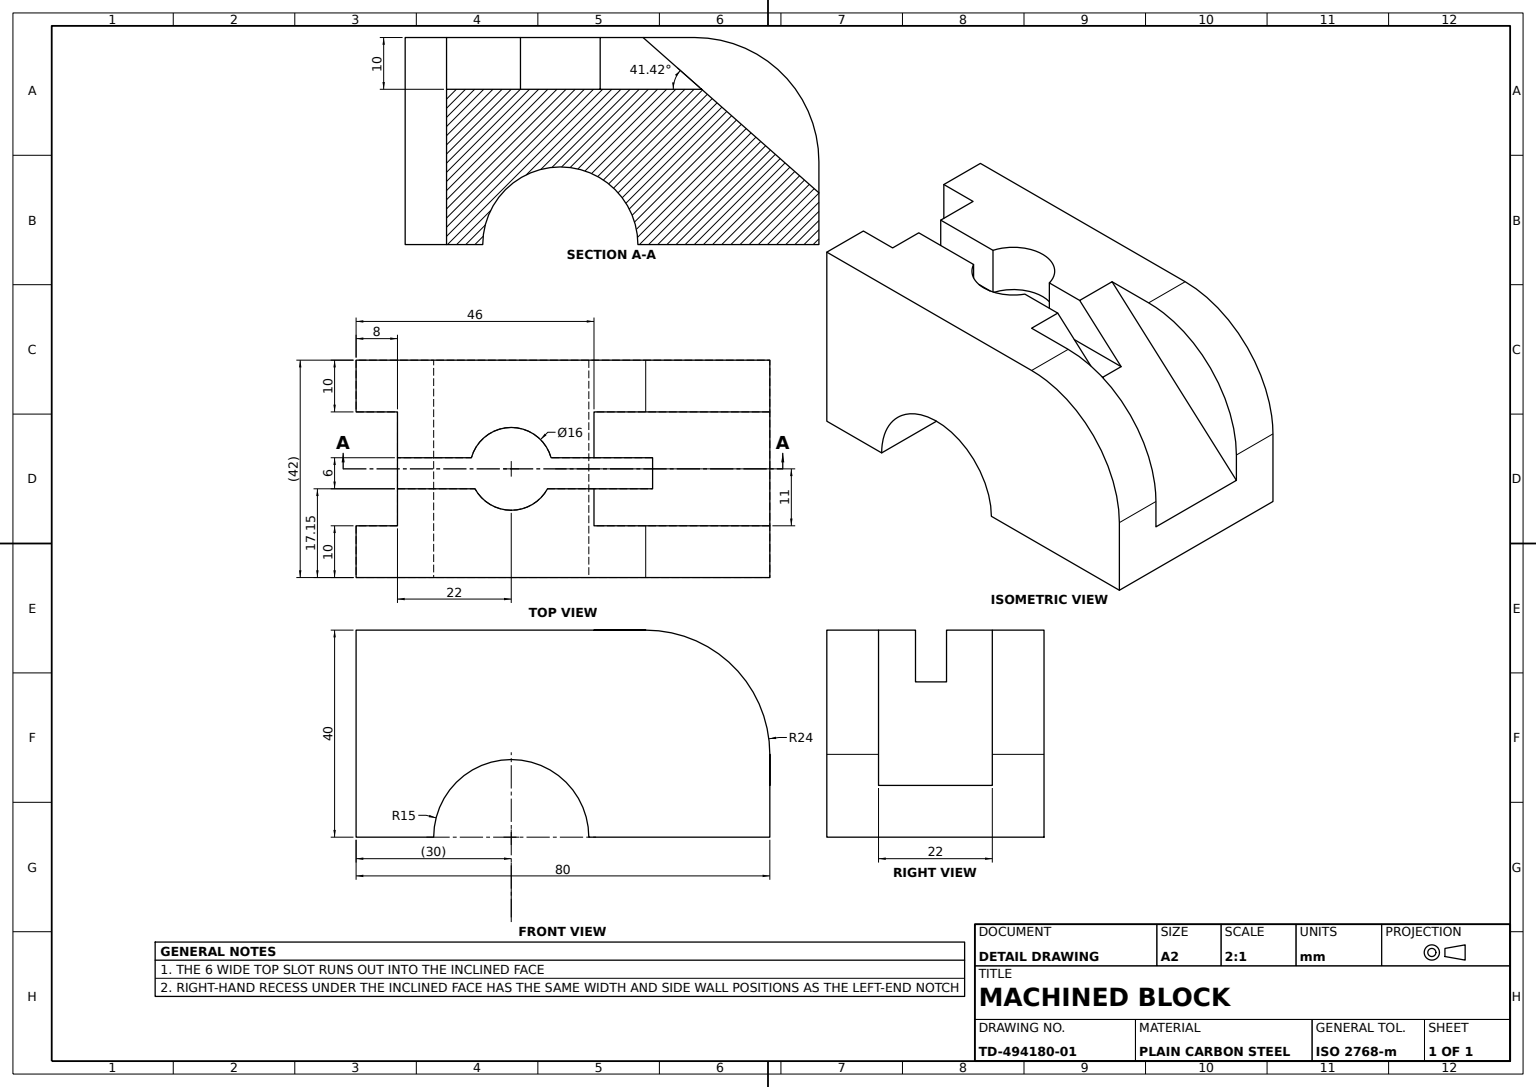
from build123d import *

# Parameters (mm, degrees)
BRACKET_BODY_DEPTH      = 42
TOP_SLOT_CUT_DEPTH      = 10
THROUGH_SLOT_10MM_DEPTH = 42
SLOT_RELIEF_SKETCH_W    = 6
SLOT_RELIEF_SKETCH_H    = 10
SLOT_RELIEF_CUT_DEPTH   = 42
SIDE_BOSS_A_SKETCH_W    = 80
SIDE_BOSS_A_SKETCH_H    = 40
SIDE_BOSS_A_DEPTH       = 10
SIDE_BOSS_B_SKETCH_W    = 80
SIDE_BOSS_B_SKETCH_H    = 40
SIDE_BOSS_B_DEPTH       = 10
CORNER_ROUND_R24_R      = 24
ARCH_CUTOUT_DEPTH       = 42
NOTCH_SKETCH_W          = 8
NOTCH_SKETCH_H          = 22
NOTCH_CUT_DEPTH         = 42


with BuildPart() as part:
    # Bracket Profile Sketch → Bracket Body (new body)
    with BuildSketch(Plane.XY):
        with BuildLine():
            Line((-40, 0), (40, 0))
            Line((40, 0), (40, 10))
            Line((40, 10), (40, 16))
            ThreePointArc((40, 16), (32.970562748, 32.970562748), (16, 40))
            Line((16, 40), (6, 40))
            Line((6, 40), (-40, 40))
            Line((-40, 40), (-40, 0))
        make_face()
    extrude(amount=-BRACKET_BODY_DEPTH)

    # Top Slot Sketch → Top Slot Cut (cut)
    with BuildSketch(Plane(origin=(0, 40, 0), x_dir=(1, 0, 0), z_dir=(0, 1, 0))):
        with BuildLine():
            Line((-40, 23.147915888), (-17.706260918, 23.147915888))
            ThreePointArc((-17.706260918, 23.147915888), (-10, 29), (-2.293739082, 23.147915888))
            Line((-2.293739082, 23.147915888), (6, 23.147915888))
            Line((6, 23.147915888), (6, 17.147915888))
            Line((6, 17.147915888), (-2.988477484, 17.147915888))
            ThreePointArc((-2.988477484, 17.147915888), (-10, 13), (-17.011522516, 17.147915888))
            Line((-17.011522516, 17.147915888), (-40, 17.147915888))
            Line((-40, 17.147915888), (-40, 23.147915888))
        make_face()
    extrude(amount=-TOP_SLOT_CUT_DEPTH, mode=Mode.SUBTRACT)

    # Through Slot Sketch → Through Slot 10mm (cut)
    with BuildSketch(Plane.XY):
        with BuildLine():
            Line((6, 40), (40, 10))
            Line((40, 10), (40, 16))
            ThreePointArc((40, 16), (32.970562748, 32.970562748), (16, 40))
            Line((16, 40), (6, 40))
        make_face()
    extrude(amount=-THROUGH_SLOT_10MM_DEPTH, mode=Mode.SUBTRACT)

    # Slot Relief Sketch → Slot Relief Cut (cut)
    with BuildSketch(Plane.ZY.offset(-6)):
        with Locations((-20.147915888, 35)):
            Rectangle(SLOT_RELIEF_SKETCH_W, SLOT_RELIEF_SKETCH_H)
    extrude(amount=-SLOT_RELIEF_CUT_DEPTH, mode=Mode.SUBTRACT)

    # Side Boss A Sketch → Side Boss A (add)
    with BuildSketch(Plane.XY):
        with Locations((0, 20)):
            Rectangle(SIDE_BOSS_A_SKETCH_W, SIDE_BOSS_A_SKETCH_H)
    extrude(amount=-SIDE_BOSS_A_DEPTH)

    # Side Boss B Sketch → Side Boss B (add)
    with BuildSketch(Plane(origin=(0, 0, -42), x_dir=(-1, 0, 0), z_dir=(0, 0, -1))):
        with Locations((0, 20)):
            Rectangle(SIDE_BOSS_B_SKETCH_W, SIDE_BOSS_B_SKETCH_H)
    extrude(amount=-SIDE_BOSS_B_DEPTH)

    # Corner Round R24
    corner_round_r24_edges = [part.edges().sort_by_distance(p)[0] for p in [
        (40, 40, -37),
        (40, 40, -5),
    ]]
    fillet(corner_round_r24_edges, radius=CORNER_ROUND_R24_R)

    # Arch Cutout Sketch → Arch Cutout (cut)
    with BuildSketch(Plane.XY):
        with BuildLine():
            Line((-25, 0), (5, 0))
            ThreePointArc((5, 0), (-10, 15), (-25, 0))
        make_face()
    extrude(amount=-ARCH_CUTOUT_DEPTH, mode=Mode.SUBTRACT)

    # Notch Sketch → Notch Cut (cut)
    with BuildSketch(Plane(origin=(0, 40, 0), x_dir=(1, 0, 0), z_dir=(0, 1, 0))):
        with Locations((-36, 21)):
            Rectangle(NOTCH_SKETCH_W, NOTCH_SKETCH_H)
    extrude(amount=-NOTCH_CUT_DEPTH, mode=Mode.SUBTRACT)


solid = part.part
